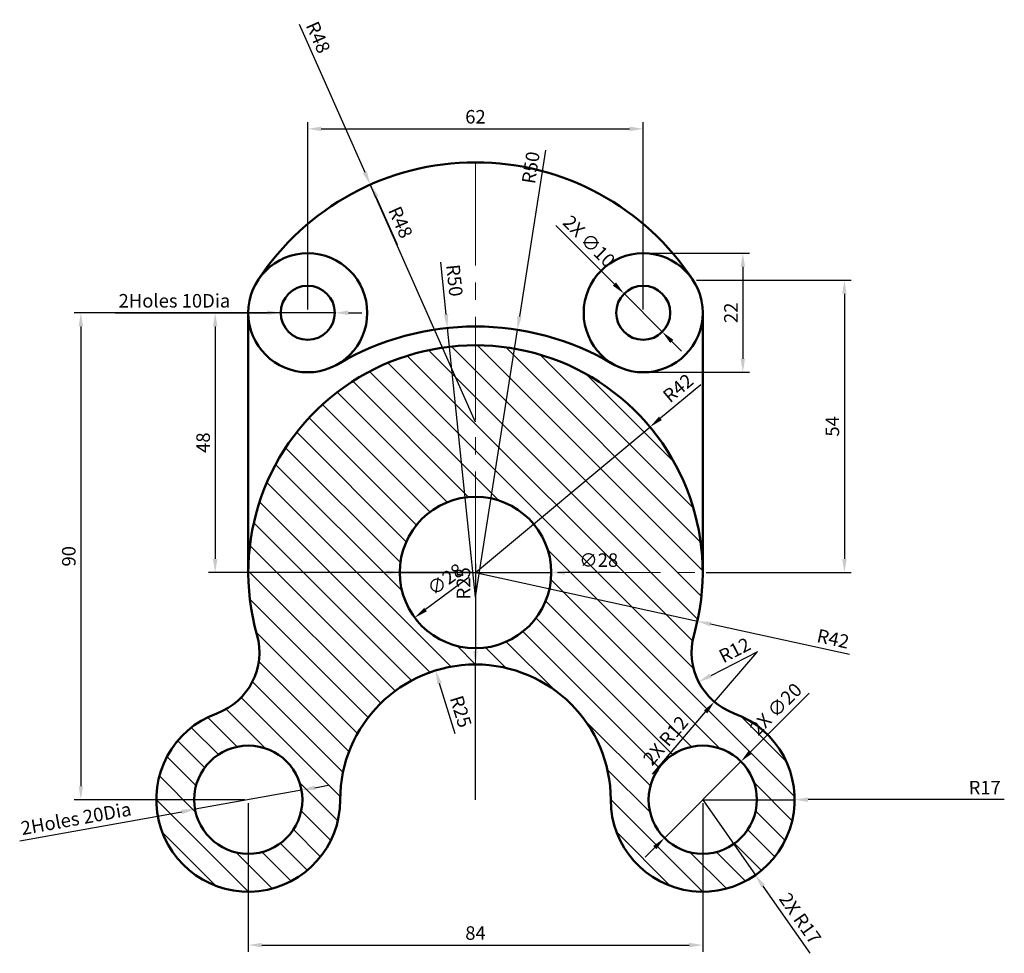
# Model space of a CAD drawing. Units: millimetres. Extents: x 9323 to 9505, y 5683 to 5855.
import ezdxf

# ---------------------------------------------------------------- set-up
doc = ezdxf.new("R2010")
doc.units = ezdxf.units.MM
doc.linetypes.add('CENTER2', pattern=[28.575, 19.05, -3.175, 3.175, -3.175])
for name, color, linetype, lineweight in [('M-CNTR', 4, 'CENTER2', 18), ('M-DIMS', 2, 'Continuous', 25), ('M-HATC', 8, 'Continuous', 18), ('M-OUTL', 7, 'Continuous', 50)]:
    doc.layers.add(name, color=color, linetype=linetype, lineweight=lineweight)
doc.styles.get("Standard").update_dxf_attribs({"font": 'arial.ttf'})
doc.dimstyles.new('ISO-25', dxfattribs={"dimtxt": 2.5, "dimasz": 2.5, "dimexe": 1.25, "dimexo": 0.625, "dimtad": 1, "dimtxsty": 'Standard', "dimcen": 2.5, "dimadec": 0, "dimazin": 0, "dimtfac": 1, "dimtmove": 0, "dimatfit": 3, "dimfxl": 1, "dimarcsym": 0})

# ---------------------------------------------------------------- blocks, each defined once
blk = doc.blocks.new('*D1')
at = {"layer": 'Defpoints', "color": 0, "transparency": 16777216}
for p in [(9449.24, 5711.15), (9466.24, 5711.16)]:
    blk.add_point(p, dxfattribs=at)
at = {"layer": 'M-DIMS', "color": 0, "lineweight": -2, "transparency": 16777216}
for p, q in [((9449.24, 5711.15), (9466.24, 5711.16)), ((9505, 5711.19), (9468.74, 5711.17))]:
    blk.add_line(p, q, dxfattribs=at)
at = {"layer": 'M-DIMS', "color": 0, "transparency": 16777216}
blk.add_solid([(9468.74, 5711.58), (9468.74, 5710.75), (9466.24, 5711.16)], dxfattribs=at)
at = {"layer": 'M-DIMS', "color": 0, "transparency": 16777216, "insert": (9501.38, 5713.07), "char_height": 2.5, "attachment_point": 5, "rotation": 0.0372}
blk.add_mtext('R17', dxfattribs=at)
blk = doc.blocks.new('*D2')
at = {"layer": 'Defpoints', "color": 0, "transparency": 16777216}
for p in [(9399.86, 5735.04), (9407.24, 5711.15)]:
    blk.add_point(p, dxfattribs=at)
at = {"layer": 'M-DIMS', "color": 0, "lineweight": -2, "transparency": 16777216}
blk.add_line((9403.48, 5723.34), (9400.6, 5732.65), dxfattribs=at)
at = {"layer": 'M-DIMS', "color": 0, "transparency": 16777216}
blk.add_solid([(9401, 5732.77), (9400.2, 5732.53), (9399.86, 5735.04)], dxfattribs=at)
at = {"layer": 'M-DIMS', "color": 0, "transparency": 16777216, "insert": (9404.22, 5727.36), "char_height": 2.5, "attachment_point": 5, "rotation": 287.1722}
blk.add_mtext('R25', dxfattribs=at)
blk = doc.blocks.new('*D3')
at = {"layer": 'Defpoints', "color": 0, "transparency": 16777216}
for p in [(9387.89, 5824.88), (9407.24, 5780.95)]:
    blk.add_point(p, dxfattribs=at)
at = {"layer": 'M-DIMS', "color": 0, "lineweight": -2, "transparency": 16777216}
blk.add_line((9392.82, 5813.69), (9388.9, 5822.59), dxfattribs=at)
at = {"layer": 'M-DIMS', "color": 0, "transparency": 16777216}
blk.add_solid([(9389.28, 5822.76), (9388.51, 5822.42), (9387.89, 5824.88)], dxfattribs=at)
at = {"layer": 'M-DIMS', "color": 0, "transparency": 16777216, "insert": (9393.1, 5817.76), "char_height": 2.5, "attachment_point": 5, "rotation": 293.7787}
blk.add_mtext('R48', dxfattribs=at)
blk = doc.blocks.new('*D4')
at = {"layer": 'Defpoints', "color": 0, "transparency": 16777216}
for p in [(9402.05, 5798.35), (9407.24, 5748.62)]:
    blk.add_point(p, dxfattribs=at)
at = {"layer": 'M-DIMS', "color": 0, "lineweight": -2, "transparency": 16777216}
for p, q in [((9400.78, 5810.5), (9401.79, 5800.83)), ((9407.24, 5748.62), (9402.05, 5798.35))]:
    blk.add_line(p, q, dxfattribs=at)
at = {"layer": 'M-DIMS', "color": 0, "transparency": 16777216}
blk.add_solid([(9402.21, 5800.88), (9401.38, 5800.79), (9402.05, 5798.35)], dxfattribs=at)
at = {"layer": 'M-DIMS', "color": 0, "transparency": 16777216, "insert": (9403.05, 5807.11), "char_height": 2.5, "attachment_point": 5, "rotation": 275.9599}
blk.add_mtext('R50', dxfattribs=at)
blk = doc.blocks.new('*D5')
at = {"layer": 'Defpoints', "color": 0, "transparency": 16777216}
for p in [(9439.5, 5780.04), (9407.24, 5753.15)]:
    blk.add_point(p, dxfattribs=at)
at = {"layer": 'M-DIMS', "color": 0, "lineweight": -2, "transparency": 16777216}
for p, q in [((9448.87, 5787.86), (9441.42, 5781.65)), ((9407.24, 5753.15), (9439.5, 5780.04))]:
    blk.add_line(p, q, dxfattribs=at)
at = {"layer": 'M-DIMS', "color": 0, "transparency": 16777216}
blk.add_solid([(9441.16, 5781.97), (9441.69, 5781.33), (9439.5, 5780.04)], dxfattribs=at)
at = {"layer": 'M-DIMS', "color": 0, "transparency": 16777216, "insert": (9444.9, 5786.99), "char_height": 2.5, "attachment_point": 5, "rotation": 39.8135}
blk.add_mtext('R42', dxfattribs=at)
blk = doc.blocks.new('*D6')
at = {"layer": 'Defpoints', "color": 0, "transparency": 16777216}
for p in [(9375.08, 5712.93), (9355.4, 5709.38)]:
    blk.add_point(p, dxfattribs=at)
at = {"layer": 'M-DIMS', "color": 0, "lineweight": -2, "transparency": 16777216}
for p, q in [((9377.54, 5713.37), (9380, 5713.82)), ((9375.08, 5712.93), (9355.4, 5709.38)), ((9322.99, 5703.53), (9352.94, 5708.93))]:
    blk.add_line(p, q, dxfattribs=at)
at = {"layer": 'M-DIMS', "color": 0, "transparency": 16777216}
for points in [[(9377.47, 5713.78), (9377.62, 5712.96), (9375.08, 5712.93)], [(9352.87, 5709.34), (9353.01, 5708.52), (9355.4, 5709.38)]]:
    blk.add_solid(points, dxfattribs=at)
at = {"layer": 'M-DIMS', "color": 0, "transparency": 16777216, "insert": (9333.46, 5707.35), "char_height": 2.5, "attachment_point": 5, "rotation": 10.2247}
blk.add_mtext('2Holes 20Dia', dxfattribs=at)
blk = doc.blocks.new('*D7')
at = {"layer": 'Defpoints', "color": 0, "transparency": 16777216}
for p in [(9418.48, 5761.5), (9396, 5744.8)]:
    blk.add_point(p, dxfattribs=at)
at = {"layer": 'M-DIMS', "color": 0, "lineweight": -2, "transparency": 16777216}
blk.add_line((9406.08, 5752.29), (9398.01, 5746.3), dxfattribs=at)
at = {"layer": 'M-DIMS', "color": 0, "transparency": 16777216}
blk.add_solid([(9397.76, 5746.63), (9398.26, 5745.96), (9396, 5744.8)], dxfattribs=at)
at = {"layer": 'M-DIMS', "color": 0, "transparency": 16777216, "insert": (9401.87, 5751.62), "char_height": 2.5, "attachment_point": 5, "rotation": 36.6061}
blk.add_mtext('∅28', dxfattribs=at)
blk = doc.blocks.new('*D8')
at = {"layer": 'Defpoints', "color": 0, "transparency": 16777216}
for p in [(9371.24, 5801.15), (9381.24, 5801.15)]:
    blk.add_point(p, dxfattribs=at)
at = {"layer": 'M-DIMS', "color": 0, "lineweight": -2, "transparency": 16777216}
for p, q in [((9340.61, 5801.15), (9368.74, 5801.15)), ((9381.24, 5801.15), (9371.24, 5801.15)), ((9383.74, 5801.15), (9386.24, 5801.15))]:
    blk.add_line(p, q, dxfattribs=at)
at = {"layer": 'M-DIMS', "color": 0, "transparency": 16777216}
for points in [[(9368.74, 5801.57), (9368.74, 5800.74), (9371.24, 5801.15)], [(9383.74, 5801.57), (9383.74, 5800.74), (9381.24, 5801.15)]]:
    blk.add_solid(points, dxfattribs=at)
at = {"layer": 'M-DIMS', "color": 0, "transparency": 16777216, "insert": (9351.59, 5803.05), "char_height": 2.5, "attachment_point": 5}
blk.add_mtext('2Holes 10Dia', dxfattribs=at)
blk = doc.blocks.new('*D9')
at = {"layer": 'Defpoints', "color": 0, "transparency": 16777216}
for p in [(9438.24, 5812.15), (9438.24, 5790.15), (9456.66, 5790.15)]:
    blk.add_point(p, dxfattribs=at)
at = {"layer": 'M-DIMS', "color": 0, "lineweight": -2, "transparency": 16777216}
for p, q in [((9438.87, 5812.15), (9457.91, 5812.15)), ((9456.66, 5809.65), (9456.66, 5792.65)), ((9438.87, 5790.15), (9457.91, 5790.15))]:
    blk.add_line(p, q, dxfattribs=at)
at = {"layer": 'M-DIMS', "color": 0, "transparency": 16777216}
for points in [[(9456.25, 5809.65), (9457.08, 5809.65), (9456.66, 5812.15)], [(9456.25, 5792.65), (9457.08, 5792.65), (9456.66, 5790.15)]]:
    blk.add_solid(points, dxfattribs=at)
at = {"layer": 'M-DIMS', "color": 0, "transparency": 16777216, "insert": (9454.78, 5801.15), "char_height": 2.5, "attachment_point": 5, "rotation": 90}
blk.add_mtext('22', dxfattribs=at)
blk = doc.blocks.new('*D10')
at = {"layer": 'Defpoints', "color": 0, "transparency": 16777216}
for p in [(9438.24, 5835.15), (9376.24, 5801.15), (9438.24, 5801.15)]:
    blk.add_point(p, dxfattribs=at)
at = {"layer": 'M-DIMS', "color": 0, "lineweight": -2, "transparency": 16777216}
for p, q in [((9376.24, 5801.78), (9376.24, 5836.4)), ((9438.24, 5801.78), (9438.24, 5836.4)), ((9378.74, 5835.15), (9435.74, 5835.15))]:
    blk.add_line(p, q, dxfattribs=at)
at = {"layer": 'M-DIMS', "color": 0, "transparency": 16777216}
for points in [[(9378.74, 5835.57), (9378.74, 5834.74), (9376.24, 5835.15)], [(9435.74, 5835.57), (9435.74, 5834.74), (9438.24, 5835.15)]]:
    blk.add_solid(points, dxfattribs=at)
at = {"layer": 'M-DIMS', "color": 0, "transparency": 16777216, "insert": (9407.24, 5837.06), "char_height": 2.5, "attachment_point": 5}
blk.add_mtext('62', dxfattribs=at)
blk = doc.blocks.new('*D11')
at = {"layer": 'Defpoints', "color": 0, "transparency": 16777216}
for p in [(9376.24, 5801.15), (9359.12, 5753.15), (9407.24, 5753.15)]:
    blk.add_point(p, dxfattribs=at)
at = {"layer": 'M-DIMS', "color": 0, "lineweight": -2, "transparency": 16777216}
for p, q in [((9375.62, 5801.15), (9357.87, 5801.15)), ((9359.12, 5798.65), (9359.12, 5755.65)), ((9406.62, 5753.15), (9357.87, 5753.15))]:
    blk.add_line(p, q, dxfattribs=at)
at = {"layer": 'M-DIMS', "color": 0, "transparency": 16777216}
for points in [[(9358.71, 5798.65), (9359.54, 5798.65), (9359.12, 5801.15)], [(9358.71, 5755.65), (9359.54, 5755.65), (9359.12, 5753.15)]]:
    blk.add_solid(points, dxfattribs=at)
at = {"layer": 'M-DIMS', "color": 0, "transparency": 16777216, "insert": (9357.22, 5777.15), "char_height": 2.5, "attachment_point": 5, "rotation": 90}
blk.add_mtext('48', dxfattribs=at)
blk = doc.blocks.new('*D12')
at = {"layer": 'Defpoints', "color": 0, "transparency": 16777216}
for p in [(9365.24, 5711.15), (9449.24, 5711.15), (9449.24, 5684.29)]:
    blk.add_point(p, dxfattribs=at)
at = {"layer": 'M-DIMS', "color": 0, "lineweight": -2, "transparency": 16777216}
for p, q in [((9365.24, 5710.53), (9365.24, 5683.04)), ((9449.24, 5710.53), (9449.24, 5683.04)), ((9367.74, 5684.29), (9446.74, 5684.29))]:
    blk.add_line(p, q, dxfattribs=at)
at = {"layer": 'M-DIMS', "color": 0, "transparency": 16777216}
for points in [[(9367.74, 5684.71), (9367.74, 5683.87), (9365.24, 5684.29)], [(9446.74, 5684.71), (9446.74, 5683.87), (9449.24, 5684.29)]]:
    blk.add_solid(points, dxfattribs=at)
at = {"layer": 'M-DIMS', "color": 0, "transparency": 16777216, "insert": (9407.24, 5686.19), "char_height": 2.5, "attachment_point": 5}
blk.add_mtext('84', dxfattribs=at)
blk = doc.blocks.new('*D13')
at = {"layer": 'Defpoints', "color": 0, "transparency": 16777216}
for p in [(9376.24, 5801.15), (9334.29, 5711.15), (9365.24, 5711.15)]:
    blk.add_point(p, dxfattribs=at)
at = {"layer": 'M-DIMS', "color": 0, "lineweight": -2, "transparency": 16777216}
for p, q in [((9375.62, 5801.15), (9333.04, 5801.15)), ((9334.29, 5798.65), (9334.29, 5713.65)), ((9364.62, 5711.15), (9333.04, 5711.15))]:
    blk.add_line(p, q, dxfattribs=at)
at = {"layer": 'M-DIMS', "color": 0, "transparency": 16777216}
for points in [[(9333.88, 5798.65), (9334.71, 5798.65), (9334.29, 5801.15)], [(9333.88, 5713.65), (9334.71, 5713.65), (9334.29, 5711.15)]]:
    blk.add_solid(points, dxfattribs=at)
at = {"layer": 'M-DIMS', "color": 0, "transparency": 16777216, "insert": (9332.39, 5756.15), "char_height": 2.5, "attachment_point": 5, "rotation": 90}
blk.add_mtext('90', dxfattribs=at)
blk = doc.blocks.new('*D14')
at = {"layer": 'Defpoints', "color": 0, "transparency": 16777216}
for p in [(9459.19, 5738.39), (9448.5, 5732.94)]:
    blk.add_point(p, dxfattribs=at)
at = {"layer": 'M-DIMS', "color": 0, "lineweight": -2, "transparency": 16777216}
blk.add_line((9459.36, 5738.48), (9450.72, 5734.08), dxfattribs=at)
at = {"layer": 'M-DIMS', "color": 0, "transparency": 16777216}
blk.add_solid([(9450.54, 5734.45), (9450.91, 5733.7), (9448.5, 5732.94)], dxfattribs=at)
at = {"layer": 'M-DIMS', "color": 0, "transparency": 16777216, "insert": (9455.3, 5738.52), "char_height": 2.5, "attachment_point": 5, "rotation": 27.0427}
blk.add_mtext('R12', dxfattribs=at)
blk = doc.blocks.new('LINK-EYE-22-10')
for radius in [11, 5]:
    blk.add_circle((11, 11), radius)
blk = doc.blocks.new('*D16')
at = {"layer": 'Defpoints', "color": 0, "transparency": 16777216}
for p in [(9447.46, 5807.16), (9449.24, 5753.15), (9475.44, 5753.15)]:
    blk.add_point(p, dxfattribs=at)
at = {"layer": 'M-DIMS', "color": 0, "lineweight": -2, "transparency": 16777216}
for p, q in [((9448.08, 5807.16), (9476.69, 5807.16)), ((9475.44, 5804.66), (9475.44, 5755.65)), ((9449.87, 5753.15), (9476.69, 5753.15))]:
    blk.add_line(p, q, dxfattribs=at)
at = {"layer": 'M-DIMS', "color": 0, "transparency": 16777216}
for points in [[(9475.02, 5804.66), (9475.85, 5804.66), (9475.44, 5807.16)], [(9475.02, 5755.65), (9475.85, 5755.65), (9475.44, 5753.15)]]:
    blk.add_solid(points, dxfattribs=at)
at = {"layer": 'M-DIMS', "color": 0, "transparency": 16777216, "insert": (9473.54, 5780.16), "char_height": 2.5, "attachment_point": 5, "rotation": 90}
blk.add_mtext('54', dxfattribs=at)
blk = doc.blocks.new('*D17')
at = {"layer": 'Defpoints', "color": 0, "transparency": 16777216}
for p in [(9387.8, 5824.84), (9407.24, 5780.95)]:
    blk.add_point(p, dxfattribs=at)
at = {"layer": 'M-DIMS', "color": 0, "lineweight": -2, "transparency": 16777216}
for p, q in [((9374.67, 5854.48), (9386.79, 5827.13)), ((9407.24, 5780.95), (9387.8, 5824.84))]:
    blk.add_line(p, q, dxfattribs=at)
at = {"layer": 'M-DIMS', "color": 0, "transparency": 16777216}
blk.add_solid([(9387.17, 5827.29), (9386.41, 5826.96), (9387.8, 5824.84)], dxfattribs=at)
at = {"layer": 'M-DIMS', "color": 0, "transparency": 16777216, "insert": (9377.87, 5851.94), "char_height": 2.5, "attachment_point": 5, "rotation": 293.8937}
blk.add_mtext('R48', dxfattribs=at)
blk = doc.blocks.new('*D18')
at = {"layer": 'Defpoints', "color": 0, "transparency": 16777216}
for p in [(9415, 5798.01), (9407.24, 5748.62)]:
    blk.add_point(p, dxfattribs=at)
at = {"layer": 'M-DIMS', "color": 0, "lineweight": -2, "transparency": 16777216}
for p, q in [((9420.21, 5831.21), (9415.39, 5800.48)), ((9407.24, 5748.62), (9415, 5798.01))]:
    blk.add_line(p, q, dxfattribs=at)
at = {"layer": 'M-DIMS', "color": 0, "transparency": 16777216}
blk.add_solid([(9414.98, 5800.55), (9415.8, 5800.42), (9415, 5798.01)], dxfattribs=at)
at = {"layer": 'M-DIMS', "color": 0, "transparency": 16777216, "insert": (9417.78, 5827.94), "char_height": 2.5, "attachment_point": 5, "rotation": 81.0736}
blk.add_mtext('R50', dxfattribs=at)
blk = doc.blocks.new('*D19')
at = {"layer": 'Defpoints', "color": 0, "transparency": 16777216}
for p in [(9407.24, 5753.15), (9448.27, 5744.15)]:
    blk.add_point(p, dxfattribs=at)
at = {"layer": 'M-DIMS', "color": 0, "lineweight": -2, "transparency": 16777216}
for p, q in [((9407.24, 5753.15), (9448.27, 5744.15)), ((9476.4, 5737.98), (9450.71, 5743.62))]:
    blk.add_line(p, q, dxfattribs=at)
at = {"layer": 'M-DIMS', "color": 0, "transparency": 16777216}
blk.add_solid([(9450.8, 5744.02), (9450.62, 5743.21), (9448.27, 5744.15)], dxfattribs=at)
at = {"layer": 'M-DIMS', "color": 0, "transparency": 16777216, "insert": (9473.28, 5740.59), "char_height": 2.5, "attachment_point": 5, "rotation": 347.6267}
blk.add_mtext('R42', dxfattribs=at)
blk = doc.blocks.new('*D20')
at = {"layer": 'Defpoints', "color": 0, "transparency": 16777216}
for p in [(9407.24, 5736.15), (9407.24, 5711.15)]:
    blk.add_point(p, dxfattribs=at)
at = {"layer": 'M-DIMS', "color": 0, "lineweight": -2, "transparency": 16777216}
for p, q in [((9407.24, 5754.77), (9407.24, 5738.65)), ((9407.24, 5711.15), (9407.24, 5736.15))]:
    blk.add_line(p, q, dxfattribs=at)
at = {"layer": 'M-DIMS', "color": 0, "transparency": 16777216}
blk.add_solid([(9406.83, 5738.65), (9407.66, 5738.65), (9407.24, 5736.15)], dxfattribs=at)
at = {"layer": 'M-DIMS', "color": 0, "transparency": 16777216, "insert": (9405.34, 5751.15), "char_height": 2.5, "attachment_point": 5, "rotation": 89.9999}
blk.add_mtext('R25', dxfattribs=at)
blk = doc.blocks.new('*D21')
at = {"layer": 'Defpoints', "color": 0, "transparency": 16777216}
for p in [(9449.24, 5711.15), (9458.99, 5697.22)]:
    blk.add_point(p, dxfattribs=at)
at = {"layer": 'M-DIMS', "color": 0, "lineweight": -2, "transparency": 16777216}
for p, q in [((9449.24, 5711.15), (9458.99, 5697.22)), ((9469.1, 5682.77), (9460.42, 5695.17))]:
    blk.add_line(p, q, dxfattribs=at)
at = {"layer": 'M-DIMS', "color": 0, "transparency": 16777216}
blk.add_solid([(9460.76, 5695.41), (9460.08, 5694.93), (9458.99, 5697.22)], dxfattribs=at)
at = {"layer": 'M-DIMS', "color": 0, "transparency": 16777216, "insert": (9467.01, 5689.03), "char_height": 2.5, "attachment_point": 5, "rotation": 304.9715}
blk.add_mtext('2X R17', dxfattribs=at)
blk = doc.blocks.new('*D22')
at = {"layer": 'Defpoints', "color": 0, "transparency": 16777216}
for p in [(9459.19, 5738.39), (9451.39, 5729.27)]:
    blk.add_point(p, dxfattribs=at)
at = {"layer": 'M-DIMS', "color": 0, "lineweight": -2, "transparency": 16777216}
for p, q in [((9459.19, 5738.39), (9451.39, 5729.27)), ((9439.96, 5715.87), (9449.77, 5727.37))]:
    blk.add_line(p, q, dxfattribs=at)
at = {"layer": 'M-DIMS', "color": 0, "transparency": 16777216}
blk.add_solid([(9449.45, 5727.64), (9450.09, 5727.1), (9451.39, 5729.27)], dxfattribs=at)
at = {"layer": 'M-DIMS', "color": 0, "transparency": 16777216, "insert": (9442.62, 5721.89), "char_height": 2.5, "attachment_point": 5, "rotation": 49.5056}
blk.add_mtext('2X R12', dxfattribs=at)
blk = doc.blocks.new('*D23')
at = {"layer": 'Defpoints', "color": 0, "transparency": 16777216}
for p in [(9393.24, 5753.15), (9421.24, 5753.15)]:
    blk.add_point(p, dxfattribs=at)
at = {"layer": 'M-DIMS', "color": 0, "lineweight": -2, "transparency": 16777216}
for p, q in [((9390.74, 5753.15), (9388.24, 5753.15)), ((9393.24, 5753.15), (9421.24, 5753.15)), ((9433.8, 5753.15), (9423.74, 5753.15))]:
    blk.add_line(p, q, dxfattribs=at)
at = {"layer": 'M-DIMS', "color": 0, "transparency": 16777216}
for points in [[(9390.74, 5753.57), (9390.74, 5752.74), (9393.24, 5753.15)], [(9423.74, 5753.57), (9423.74, 5752.74), (9421.24, 5753.15)]]:
    blk.add_solid(points, dxfattribs=at)
at = {"layer": 'M-DIMS', "color": 0, "transparency": 16777216, "insert": (9430.02, 5755.12), "char_height": 2.5, "attachment_point": 5, "rotation": 0.0014}
blk.add_mtext('∅28', dxfattribs=at)
blk = doc.blocks.new('*D24')
at = {"layer": 'Defpoints', "color": 0, "transparency": 16777216}
for p in [(9456.31, 5718.22), (9442.17, 5704.08)]:
    blk.add_point(p, dxfattribs=at)
at = {"layer": 'M-DIMS', "color": 0, "lineweight": -2, "transparency": 16777216}
for p, q in [((9468.92, 5730.83), (9458.08, 5719.99)), ((9442.17, 5704.08), (9456.31, 5718.22)), ((9440.4, 5702.31), (9438.63, 5700.55))]:
    blk.add_line(p, q, dxfattribs=at)
at = {"layer": 'M-DIMS', "color": 0, "transparency": 16777216}
for points in [[(9457.79, 5720.29), (9458.38, 5719.7), (9456.31, 5718.22)], [(9440.11, 5702.61), (9440.7, 5702.02), (9442.17, 5704.08)]]:
    blk.add_solid(points, dxfattribs=at)
at = {"layer": 'M-DIMS', "color": 0, "transparency": 16777216, "insert": (9462.99, 5727.69), "char_height": 2.5, "attachment_point": 5, "rotation": 44.9972}
blk.add_mtext('2X ∅20', dxfattribs=at)
blk = doc.blocks.new('*D25')
at = {"layer": 'Defpoints', "color": 0, "transparency": 16777216}
for p in [(9434.7, 5804.69), (9441.78, 5797.62)]:
    blk.add_point(p, dxfattribs=at)
at = {"layer": 'M-DIMS', "color": 0, "lineweight": -2, "transparency": 16777216}
for p, q in [((9422.09, 5817.28), (9432.94, 5806.45)), ((9441.78, 5797.62), (9434.7, 5804.69)), ((9443.55, 5795.85), (9445.32, 5794.09))]:
    blk.add_line(p, q, dxfattribs=at)
at = {"layer": 'M-DIMS', "color": 0, "transparency": 16777216}
for points in [[(9433.23, 5806.75), (9432.64, 5806.16), (9434.7, 5804.69)], [(9443.84, 5796.15), (9443.25, 5795.56), (9441.78, 5797.62)]]:
    blk.add_solid(points, dxfattribs=at)
at = {"layer": 'M-DIMS', "color": 0, "transparency": 16777216, "insert": (9428.02, 5814.14), "char_height": 2.5, "attachment_point": 5, "rotation": 315.0374}
blk.add_mtext('2X ∅10', dxfattribs=at)

msp = doc.modelspace()

# ---------------------------------------------------------------- hatches: boundary and pattern name
at = {"layer": 'M-HATC', "transparency": 33554551}
h = msp.add_hatch(dxfattribs=at)
h.set_pattern_fill('ANSI31', color=256, scale=1.1, angle=90)
h.paths.add_polyline_path([(9407.242, 5767.153), (9407.242, 5795.153, 0.4142136), (9365.242, 5753.153), (9393.242, 5753.153, -0.4142136)])
h.paths.add_polyline_path([(9407.242, 5739.153, -0.4142136), (9393.242, 5753.153), (9365.242, 5753.153, 0.0693163), (9366.841, 5741.674, -0.392938), (9359.413, 5727.122, 1.9198825), (9382.242, 5711.153, -0.4142136), (9407.242, 5736.153)])
h.paths.add_polyline_path([(9375.242, 5711.153, -1), (9355.242, 5711.153, -1)], flags=16)
h.paths.add_polyline_path([(9407.242, 5795.153), (9407.242, 5767.153, -0.4142136), (9421.242, 5753.153), (9449.242, 5753.153, 0.4142136)])
h.paths.add_polyline_path([(9447.643, 5741.674, 0.0693163), (9449.242, 5753.153), (9421.242, 5753.153, -0.4142136), (9407.242, 5739.153), (9407.242, 5736.153, -0.4142136), (9432.242, 5711.153, 1.9198825), (9455.071, 5727.122, -0.392938)])
h.paths.add_polyline_path([(9459.242, 5711.153, -1), (9439.242, 5711.153, -1)], flags=16)

# ---------------------------------------------------------------- linework, layer by layer
at = {"layer": 'M-CNTR'}
for p, q in [((9407.242, 5828.954), (9407.242, 5736.153)), ((9365.242, 5753.153), (9449.242, 5753.153))]:
    msp.add_line(p, q, dxfattribs=at)
at = {"layer": 'M-OUTL'}
for p, q in [((9365.242, 5801.153), (9365.242, 5753.153)), ((9449.242, 5801.153), (9449.242, 5753.153))]:
    msp.add_line(p, q, dxfattribs=at)
for centre, radius in [((9407.242, 5753.153), 14), ((9365.242, 5711.153), 10), ((9449.242, 5711.153), 10)]:
    msp.add_circle(centre, radius, dxfattribs=at)
for centre, radius, start, end in [((9407.242, 5780.954), 48, 33.0875, 146.9125), ((9407.242, 5748.617), 50, 59.45621, 120.54379), ((9407.242, 5753.153), 42, 344.13923, 195.86077), ((9355.298, 5738.394), 12, 290.05376, 15.86077), ((9459.186, 5738.394), 12, 164.13923, 249.94624), ((9407.242, 5711.153), 25, 0, 180), ((9365.242, 5711.153), 17, 110.05376, 0), ((9449.242, 5711.153), 17, 180, 69.94624)]:
    msp.add_arc(centre, radius, start, end, dxfattribs=at)

# ---------------------------------------------------------------- block references
for p in [(9365.242, 5790.153), (9427.242, 5790.153)]:
    msp.add_blockref('LINK-EYE-22-10', p, dxfattribs=at)

# ---------------------------------------------------------------- dimensions: what is measured, and where the dimension line sits
at = {"layer": 'M-DIMS'}
for center, mpoint, override, picture, middle in [((9407.242, 5780.954), (9387.8, 5824.84), {"dimdec": 0, "dimlfac": 1, "dimrnd": 0, "dimzin": 0, "dimdsep": 46, "dimlunit": 2}, '*D17', (9376.135, 5851.172)), ((9407.242, 5748.617), (9415, 5798.011), {"dimdec": 0, "dimlfac": 1, "dimrnd": 0, "dimzin": 0, "dimdsep": 46, "dimlunit": 2}, '*D18', (9419.655, 5827.648)), ((9407.242, 5780.954), (9387.888, 5824.879), {"dimclrd": 0, "dimclre": 0, "dimclrt": 0}, '*D3', (9391.361, 5816.996)), ((9407.242, 5711.153), (9407.242, 5736.153), {"dimdec": 0, "dimlfac": 1, "dimrnd": 0, "dimzin": 0, "dimdsep": 46, "dimlunit": 2}, '*D20', (9407.242, 5751.153)), ((9407.242, 5753.153), (9448.266, 5744.153), {"dimdec": 0, "dimlfac": 1, "dimrnd": 0, "dimzin": 0, "dimdsep": 46, "dimlunit": 2}, '*D19', (9472.881, 5738.753)), ((9459.186, 5738.394), (9448.498, 5732.939), {"dimclrd": 0, "dimclre": 0, "dimclrt": 0}, '*D14', (9456.157, 5736.848)), ((9407.242, 5711.153), (9399.861, 5735.038), {"dimclrd": 0, "dimclre": 0, "dimclrt": 0}, '*D2', (9402.406, 5726.801)), ((9449.242, 5711.153), (9466.242, 5711.164), {"dimclrd": 0, "dimclre": 0, "dimclrt": 0}, '*D1', (9501.386, 5711.187))]:
    dim = msp.add_radius_dim(center=center, mpoint=mpoint, dimstyle='ISO-25', override=override, dxfattribs=at)
    dim.commit()
    dim.dimension.update_dxf_attribs({"geometry": picture, "text_midpoint": middle, "dimtype": 164})
for base, p1, p2, picture, middle in [((9438.242, 5835.154), (9376.242, 5801.153), (9438.242, 5801.153), '*D10', (9407.242, 5837.055)), ((9449.242, 5684.291), (9365.242, 5711.153), (9449.242, 5711.153), '*D12', (9407.242, 5686.193))]:
    dim = msp.add_linear_dim(base=base, p1=p1, p2=p2, dimstyle='ISO-25', override={"dimclrd": 0, "dimclre": 0, "dimclrt": 0}, dxfattribs=at)
    dim.commit()
    dim.dimension.update_dxf_attribs({"geometry": picture, "text_midpoint": middle})
dim = msp.add_diameter_dim_2p(p1=(9441.78, 5797.619), p2=(9434.704, 5804.686), text='2X <>', dimstyle='ISO-25', override={"dimdec": 0, "dimlfac": 1, "dimrnd": 0, "dimzin": 0, "dimdsep": 46, "dimlunit": 2}, dxfattribs=at)
dim.commit()
dim.dimension.update_dxf_attribs({"geometry": '*D25', "text_midpoint": (9426.629, 5812.75)})
for base, p1, p2, override, picture, middle in [((9456.663, 5790.153), (9438.242, 5812.153), (9438.242, 5790.153), {"dimclrd": 0, "dimclre": 0, "dimclrt": 0}, '*D9', (9454.783, 5801.153)), ((9475.438, 5753.153), (9447.458, 5807.158), (9449.242, 5753.153), {"dimdec": 0, "dimlfac": 1, "dimrnd": 0, "dimzin": 0, "dimdsep": 46, "dimlunit": 2}, '*D16', (9473.542, 5780.155)), ((9334.293, 5711.153), (9376.242, 5801.153), (9365.242, 5711.153), {"dimclrd": 0, "dimclre": 0, "dimclrt": 0}, '*D13', (9332.392, 5756.153)), ((9359.124, 5753.153), (9376.242, 5801.153), (9407.242, 5753.153), {"dimclrd": 0, "dimclre": 0, "dimclrt": 0}, '*D11', (9357.223, 5777.153))]:
    dim = msp.add_linear_dim(base=base, p1=p1, p2=p2, angle=90, dimstyle='ISO-25', override=override, dxfattribs=at)
    dim.commit()
    dim.dimension.update_dxf_attribs({"geometry": picture, "text_midpoint": middle})
for center, mpoint, picture, middle in [((9407.242, 5748.617), (9402.05, 5798.347), '*D4', (9403.048, 5807.105)), ((9407.242, 5753.153), (9439.504, 5780.045), '*D5', (9444.905, 5786.995))]:
    dim = msp.add_radius_dim(center=center, mpoint=mpoint, dimstyle='ISO-25', override={"dimclrd": 0, "dimclre": 0, "dimclrt": 0}, dxfattribs=at)
    dim.commit()
    dim.dimension.update_dxf_attribs({"geometry": picture, "text_midpoint": middle})
for p1, p2, text, override, picture, middle in [((9381.242, 5801.153), (9371.242, 5801.153), '2Holes 10Dia', {"dimclrd": 0, "dimclre": 0, "dimclrt": 0}, '*D8', (9351.59, 5801.153)), ((9442.171, 5704.082), (9456.313, 5718.223), '2X <>', {"dimdec": 0, "dimlfac": 1, "dimrnd": 0, "dimzin": 0, "dimdsep": 46, "dimlunit": 2}, '*D24', (9464.383, 5726.292)), ((9375.083, 5712.928), (9355.401, 5709.378), '2Holes 20Dia', {"dimclrd": 0, "dimclre": 0, "dimclrt": 0}, '*D6', (9333.795, 5705.481))]:
    dim = msp.add_diameter_dim_2p(p1=p1, p2=p2, text=text, dimstyle='ISO-25', override=override, dxfattribs=at)
    dim.commit()
    dim.dimension.update_dxf_attribs({"geometry": picture, "text_midpoint": middle, "dimtype": 163})
for p1, p2, override, picture, middle in [((9418.481, 5761.501), (9396.003, 5744.804), {"dimclrd": 0, "dimclre": 0, "dimclrt": 0}, '*D7', (9403.05, 5750.039)), ((9393.242, 5753.152), (9421.242, 5753.153), {"dimdec": 0, "dimlfac": 1, "dimrnd": 0, "dimzin": 0, "dimdsep": 46, "dimlunit": 2}, '*D23', (9430.02, 5753.153))]:
    dim = msp.add_diameter_dim_2p(p1=p1, p2=p2, dimstyle='ISO-25', override=override, dxfattribs=at)
    dim.commit()
    dim.dimension.update_dxf_attribs({"geometry": picture, "text_midpoint": middle, "dimtype": 163})
for center, mpoint, picture, middle in [((9459.186, 5738.394), (9451.394, 5729.269), '*D22', (9442.621, 5721.892)), ((9449.242, 5711.153), (9458.986, 5697.222), '*D21', (9467.015, 5689.025))]:
    dim = msp.add_radius_dim(center=center, mpoint=mpoint, text='2X <>', dimstyle='ISO-25', override={"dimdec": 0, "dimlfac": 1, "dimrnd": 0, "dimzin": 0, "dimdsep": 46, "dimlunit": 2}, dxfattribs=at)
    dim.commit()
    dim.dimension.update_dxf_attribs({"geometry": picture, "text_midpoint": middle})

doc.saveas('drawing.dxf')
